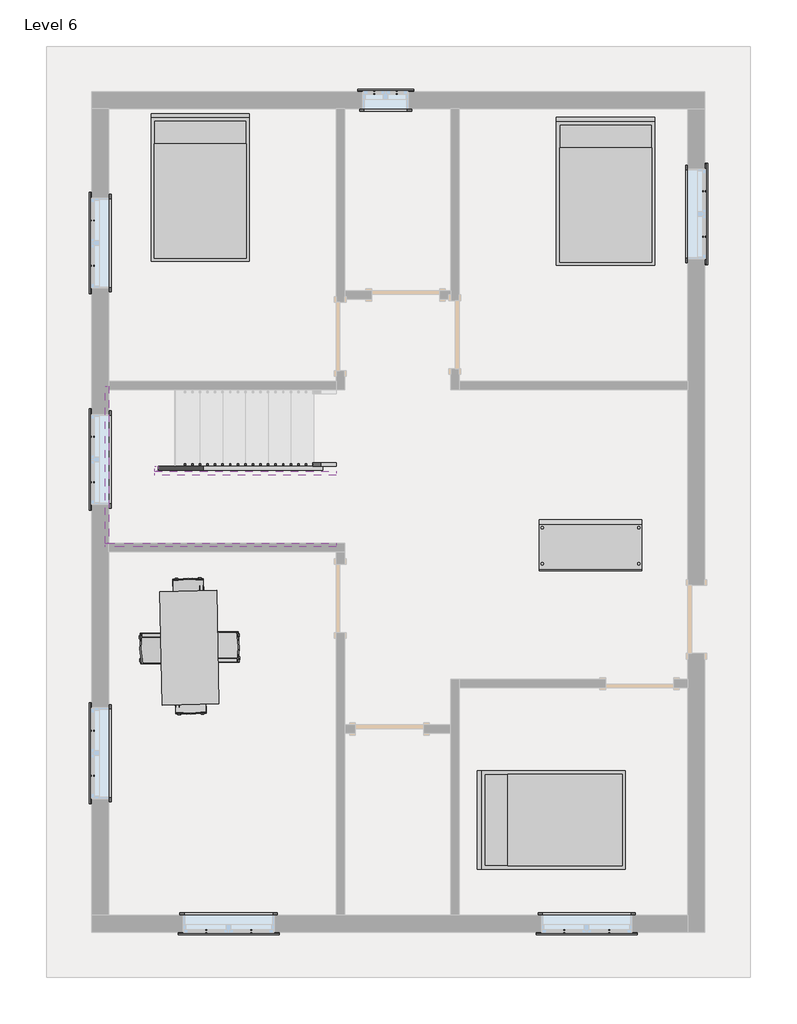
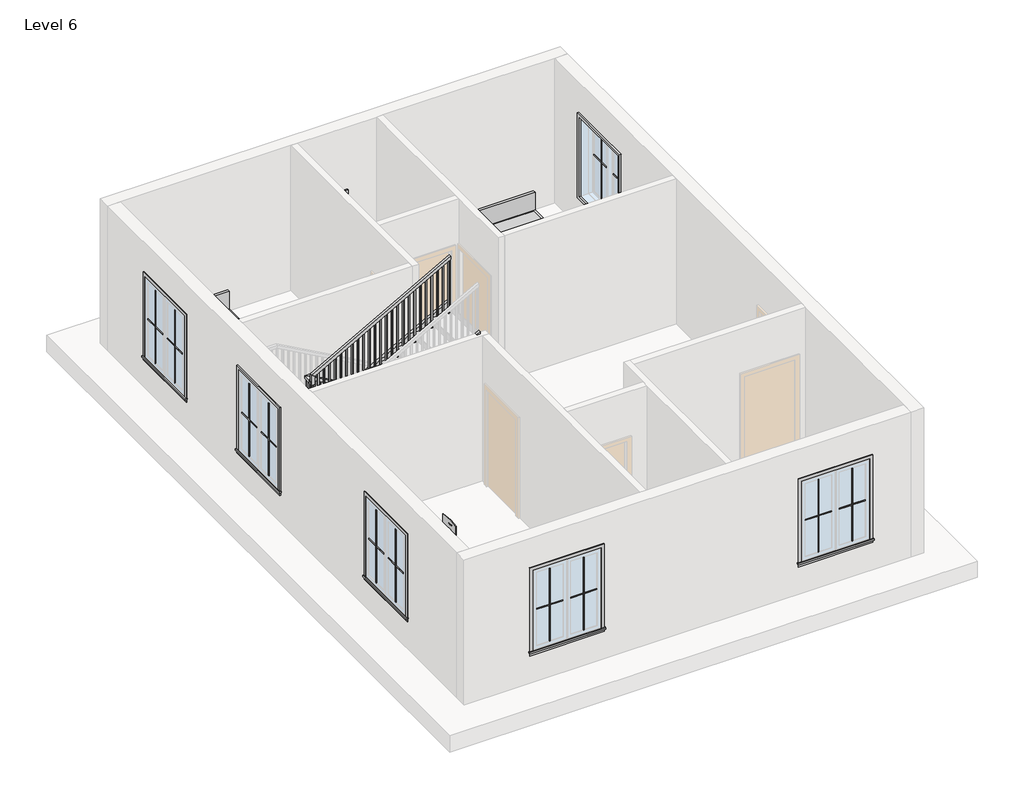
# One storey, part 2 of 2: 29 proxies, 6 members, 4 furniture elements, 1 railing.
"""IFC4 building model written with IfcOpenShell, lengths in millimetres."""

from ifc_helpers import new_model, si_unit, frame, origin, place, context, project, spatial, polyline, outline, extrude, faceted_brep, transform, mapped, element, save
from components import modern_coffee_table_17989_modern_coffee_table_17989_d3a860c8, muntin_pattern_2x2_muntin_pattern_2x2_6dad3731, muntin_pattern_2x2_muntin_pattern_2x2_a30a3345, muntin_pattern_2x2_muntin_pattern_2x2_53152e2c, muntin_pattern_2x2_muntin_pattern_2x2_e8f3e573, trim_window_exterior_flat_with_sill_92b9b949, trim_window_exterior_flat_with_sill_a665a915, trim_window_interior_flat_picture_frame_3bb882cf, trim_window_interior_flat_picture_frame_d485c387, bed_17739_bed_17739_15c61121, dining_table_w_chairs_11374_0cdfc61b

model = new_model("IFC4")

# Units and contexts
model_context = context("Model", 3, world=origin())
ifc_project = project(units=[si_unit("LENGTHUNIT", "METRE", prefix="MILLI")], contexts=[model_context])

# Site, building, storey
site = spatial("IfcSite", under=ifc_project)
building = spatial("IfcBuilding", under=site)
storey = spatial("IfcBuildingStorey", under=building, Name="Level 6", Elevation=15240.0)

# Proxies
placement = place(None, origin())
modern_coffee_table_17989_modern_coffee_table_17989_shape = modern_coffee_table_17989_modern_coffee_table_17989_d3a860c8(model_context)
element("IfcBuildingElementProxy", 1, Name="Modern_Coffee_Table_17989 : Modern_Coffee_Table_17989", ObjectType="Modern_Coffee_Table_17989 : Modern_Coffee_Table_17989", at=placement, inside=storey, context=model_context, shape_type="MappedRepresentation", body=[
    mapped(modern_coffee_table_17989_modern_coffee_table_17989_shape, transform((7937.5, 8234.1992646, 15240.0), x_axis=(1.0, 0.0, 0.0), y_axis=(0.0, 1.0, 0.0), z_axis=(0.0, 0.0, 1.0))),
])
muntin_pattern_2x2_muntin_pattern_2x2_shape = muntin_pattern_2x2_muntin_pattern_2x2_6dad3731(model_context)
element("IfcBuildingElementProxy", 2, Name="Muntin Pattern_2x2 : Muntin Pattern_2x2", ObjectType="Muntin Pattern_2x2 : Muntin Pattern_2x2", at=placement, inside=storey, context=model_context, shape_type="MappedRepresentation", body=[
    mapped(muntin_pattern_2x2_muntin_pattern_2x2_shape, transform((7961.3125, 2701.925, 16224.25), x_axis=(-1.0, 0.0, 0.0), y_axis=(0.0, -1.0, 0.0), z_axis=(0.0, 0.0, 1.0))),
])
element("IfcBuildingElementProxy", 3, Name="Muntin Pattern_2x2 : Muntin Pattern_2x2", ObjectType="Muntin Pattern_2x2 : Muntin Pattern_2x2", at=placement, inside=storey, context=model_context, shape_type="MappedRepresentation", body=[
    mapped(muntin_pattern_2x2_muntin_pattern_2x2_shape, transform((3154.3625, 2701.925, 16224.25), x_axis=(-1.0, 0.0, 0.0), y_axis=(0.0, -1.0, 0.0), z_axis=(0.0, 0.0, 1.0))),
])
element("IfcBuildingElementProxy", 4, Name="Muntin Pattern_2x2 : Muntin Pattern_2x2", ObjectType="Muntin Pattern_2x2 : Muntin Pattern_2x2", at=placement, inside=storey, context=model_context, shape_type="MappedRepresentation", body=[
    mapped(muntin_pattern_2x2_muntin_pattern_2x2_shape, transform((1025.525, 4789.4875, 16224.25), x_axis=(0.0, 1.0, 0.0), y_axis=(-1.0, 0.0, 0.0), z_axis=(0.0, 0.0, 1.0))),
])
element("IfcBuildingElementProxy", 5, Name="Muntin Pattern_2x2 : Muntin Pattern_2x2", ObjectType="Muntin Pattern_2x2 : Muntin Pattern_2x2", at=placement, inside=storey, context=model_context, shape_type="MappedRepresentation", body=[
    mapped(muntin_pattern_2x2_muntin_pattern_2x2_shape, transform((1025.525, 8732.8375, 16224.25), x_axis=(0.0, 1.0, 0.0), y_axis=(-1.0, 0.0, 0.0), z_axis=(0.0, 0.0, 1.0))),
])
element("IfcBuildingElementProxy", 6, Name="Muntin Pattern_2x2 : Muntin Pattern_2x2", ObjectType="Muntin Pattern_2x2 : Muntin Pattern_2x2", at=placement, inside=storey, context=model_context, shape_type="MappedRepresentation", body=[
    mapped(muntin_pattern_2x2_muntin_pattern_2x2_shape, transform((1025.525, 11637.9625, 16224.25), x_axis=(0.0, 1.0, 0.0), y_axis=(-1.0, 0.0, 0.0), z_axis=(0.0, 0.0, 1.0))),
])
element("IfcBuildingElementProxy", 7, Name="Muntin Pattern_2x2 : Muntin Pattern_2x2", ObjectType="Muntin Pattern_2x2 : Muntin Pattern_2x2", at=placement, inside=storey, context=model_context, shape_type="MappedRepresentation", body=[
    mapped(muntin_pattern_2x2_muntin_pattern_2x2_shape, transform((9236.075, 12634.9125, 16224.25), x_axis=(0.0, -1.0, 0.0), y_axis=(1.0, 0.0, 0.0), z_axis=(0.0, 0.0, 1.0))),
])
muntin_pattern_2x2_muntin_pattern_2x2_2_shape = muntin_pattern_2x2_muntin_pattern_2x2_a30a3345(model_context)
element("IfcBuildingElementProxy", 8, Name="Muntin Pattern_2x2 : Muntin Pattern_2x2", ObjectType="Muntin Pattern_2x2 : Muntin Pattern_2x2", at=placement, inside=storey, context=model_context, shape_type="MappedRepresentation", body=[
    mapped(muntin_pattern_2x2_muntin_pattern_2x2_2_shape, transform((7354.8875, 2701.925, 16224.25), x_axis=(1.0, 0.0, 0.0), y_axis=(0.0, 1.0, 0.0), z_axis=(0.0, 0.0, 1.0))),
])
element("IfcBuildingElementProxy", 9, Name="Muntin Pattern_2x2 : Muntin Pattern_2x2", ObjectType="Muntin Pattern_2x2 : Muntin Pattern_2x2", at=placement, inside=storey, context=model_context, shape_type="MappedRepresentation", body=[
    mapped(muntin_pattern_2x2_muntin_pattern_2x2_2_shape, transform((2547.9375, 2701.925, 16224.25), x_axis=(1.0, 0.0, 0.0), y_axis=(0.0, 1.0, 0.0), z_axis=(0.0, 0.0, 1.0))),
])
element("IfcBuildingElementProxy", 10, Name="Muntin Pattern_2x2 : Muntin Pattern_2x2", ObjectType="Muntin Pattern_2x2 : Muntin Pattern_2x2", at=placement, inside=storey, context=model_context, shape_type="MappedRepresentation", body=[
    mapped(muntin_pattern_2x2_muntin_pattern_2x2_2_shape, transform((1025.525, 5395.9125, 16224.25), x_axis=(0.0, -1.0, 0.0), y_axis=(1.0, 0.0, 0.0), z_axis=(0.0, 0.0, 1.0))),
])
element("IfcBuildingElementProxy", 11, Name="Muntin Pattern_2x2 : Muntin Pattern_2x2", ObjectType="Muntin Pattern_2x2 : Muntin Pattern_2x2", at=placement, inside=storey, context=model_context, shape_type="MappedRepresentation", body=[
    mapped(muntin_pattern_2x2_muntin_pattern_2x2_2_shape, transform((1025.525, 9339.2625, 16224.25), x_axis=(0.0, -1.0, 0.0), y_axis=(1.0, 0.0, 0.0), z_axis=(0.0, 0.0, 1.0))),
])
element("IfcBuildingElementProxy", 12, Name="Muntin Pattern_2x2 : Muntin Pattern_2x2", ObjectType="Muntin Pattern_2x2 : Muntin Pattern_2x2", at=placement, inside=storey, context=model_context, shape_type="MappedRepresentation", body=[
    mapped(muntin_pattern_2x2_muntin_pattern_2x2_2_shape, transform((1025.525, 12244.3875, 16224.25), x_axis=(0.0, -1.0, 0.0), y_axis=(1.0, 0.0, 0.0), z_axis=(0.0, 0.0, 1.0))),
])
element("IfcBuildingElementProxy", 13, Name="Muntin Pattern_2x2 : Muntin Pattern_2x2", ObjectType="Muntin Pattern_2x2 : Muntin Pattern_2x2", at=placement, inside=storey, context=model_context, shape_type="MappedRepresentation", body=[
    mapped(muntin_pattern_2x2_muntin_pattern_2x2_2_shape, transform((9236.075, 12028.4875, 16224.25), x_axis=(0.0, 1.0, 0.0), y_axis=(-1.0, 0.0, 0.0), z_axis=(0.0, 0.0, 1.0))),
])
muntin_pattern_2x2_muntin_pattern_2x2_3_shape = muntin_pattern_2x2_muntin_pattern_2x2_53152e2c(model_context)
element("IfcBuildingElementProxy", 14, Name="Muntin Pattern_2x2 : Muntin Pattern_2x2", ObjectType="Muntin Pattern_2x2 : Muntin Pattern_2x2", at=placement, inside=storey, context=model_context, shape_type="MappedRepresentation", body=[
    mapped(muntin_pattern_2x2_muntin_pattern_2x2_3_shape, transform((4808.5375, 13960.475, 16224.25), x_axis=(1.0, 0.0, 0.0), y_axis=(0.0, 1.0, 0.0), z_axis=(0.0, 0.0, 1.0))),
])
muntin_pattern_2x2_muntin_pattern_2x2_4_shape = muntin_pattern_2x2_muntin_pattern_2x2_e8f3e573(model_context)
element("IfcBuildingElementProxy", 15, Name="Muntin Pattern_2x2 : Muntin Pattern_2x2", ObjectType="Muntin Pattern_2x2 : Muntin Pattern_2x2", at=placement, inside=storey, context=model_context, shape_type="MappedRepresentation", body=[
    mapped(muntin_pattern_2x2_muntin_pattern_2x2_4_shape, transform((5110.1625, 13960.475, 16224.25), x_axis=(-1.0, 0.0, 0.0), y_axis=(0.0, -1.0, 0.0), z_axis=(0.0, 0.0, 1.0))),
])
trim_window_exterior_flat_with_sill_shape = trim_window_exterior_flat_with_sill_92b9b949(model_context)
element("IfcBuildingElementProxy", 16, Name="Trim-Window-Exterior-Flat : with Sill", ObjectType="Trim-Window-Exterior-Flat : with Sill", at=placement, inside=storey, context=model_context, shape_type="MappedRepresentation", body=[
    mapped(trim_window_exterior_flat_with_sill_shape, transform((7658.1, 2692.4, 17678.4), x_axis=(1.0, 0.0, 0.0), y_axis=(0.0, 0.0, 1.0), z_axis=(0.0, -1.0, 0.0))),
])
element("IfcBuildingElementProxy", 17, Name="Trim-Window-Exterior-Flat : with Sill", ObjectType="Trim-Window-Exterior-Flat : with Sill", at=placement, inside=storey, context=model_context, shape_type="MappedRepresentation", body=[
    mapped(trim_window_exterior_flat_with_sill_shape, transform((2851.15, 2692.4, 17678.4), x_axis=(1.0, 0.0, 0.0), y_axis=(0.0, 0.0, 1.0), z_axis=(0.0, -1.0, 0.0))),
])
element("IfcBuildingElementProxy", 18, Name="Trim-Window-Exterior-Flat : with Sill", ObjectType="Trim-Window-Exterior-Flat : with Sill", at=placement, inside=storey, context=model_context, shape_type="MappedRepresentation", body=[
    mapped(trim_window_exterior_flat_with_sill_shape, transform((1016.0, 5092.7, 17678.4), x_axis=(0.0, -1.0, 0.0), y_axis=(0.0, 0.0, 1.0), z_axis=(-1.0, 0.0, 0.0))),
])
element("IfcBuildingElementProxy", 19, Name="Trim-Window-Exterior-Flat : with Sill", ObjectType="Trim-Window-Exterior-Flat : with Sill", at=placement, inside=storey, context=model_context, shape_type="MappedRepresentation", body=[
    mapped(trim_window_exterior_flat_with_sill_shape, transform((1016.0, 9036.05, 17678.4), x_axis=(0.0, -1.0, 0.0), y_axis=(0.0, 0.0, 1.0), z_axis=(-1.0, 0.0, 0.0))),
])
element("IfcBuildingElementProxy", 20, Name="Trim-Window-Exterior-Flat : with Sill", ObjectType="Trim-Window-Exterior-Flat : with Sill", at=placement, inside=storey, context=model_context, shape_type="MappedRepresentation", body=[
    mapped(trim_window_exterior_flat_with_sill_shape, transform((1016.0, 11941.175, 17678.4), x_axis=(0.0, -1.0, 0.0), y_axis=(0.0, 0.0, 1.0), z_axis=(-1.0, 0.0, 0.0))),
])
element("IfcBuildingElementProxy", 21, Name="Trim-Window-Exterior-Flat : with Sill", ObjectType="Trim-Window-Exterior-Flat : with Sill", at=placement, inside=storey, context=model_context, shape_type="MappedRepresentation", body=[
    mapped(trim_window_exterior_flat_with_sill_shape, transform((9245.6, 12331.7, 17678.4), x_axis=(0.0, 1.0, 0.0), y_axis=(0.0, 0.0, 1.0), z_axis=(1.0, 0.0, 0.0))),
])
trim_window_exterior_flat_with_sill_2_shape = trim_window_exterior_flat_with_sill_a665a915(model_context)
element("IfcBuildingElementProxy", 22, Name="Trim-Window-Exterior-Flat : with Sill", ObjectType="Trim-Window-Exterior-Flat : with Sill", at=placement, inside=storey, context=model_context, shape_type="MappedRepresentation", body=[
    mapped(trim_window_exterior_flat_with_sill_2_shape, transform((4959.35, 13970.0, 17068.8), x_axis=(-1.0, 0.0, 0.0), y_axis=(0.0, 0.0, 1.0), z_axis=(0.0, 1.0, 0.0))),
])
trim_window_interior_flat_picture_frame_shape = trim_window_interior_flat_picture_frame_3bb882cf(model_context)
element("IfcBuildingElementProxy", 23, Name="Trim-Window-Interior-Flat : Picture Frame", ObjectType="Trim-Window-Interior-Flat : Picture Frame", at=placement, inside=storey, context=model_context, shape_type="MappedRepresentation", body=[
    mapped(trim_window_interior_flat_picture_frame_shape, transform((7658.1, 2921.0, 17678.4), x_axis=(-1.0, 0.0, 0.0), y_axis=(0.0, 0.0, 1.0), z_axis=(0.0, 1.0, 0.0))),
])
element("IfcBuildingElementProxy", 24, Name="Trim-Window-Interior-Flat : Picture Frame", ObjectType="Trim-Window-Interior-Flat : Picture Frame", at=placement, inside=storey, context=model_context, shape_type="MappedRepresentation", body=[
    mapped(trim_window_interior_flat_picture_frame_shape, transform((2851.15, 2921.0, 17678.4), x_axis=(-1.0, 0.0, 0.0), y_axis=(0.0, 0.0, 1.0), z_axis=(0.0, 1.0, 0.0))),
])
element("IfcBuildingElementProxy", 25, Name="Trim-Window-Interior-Flat : Picture Frame", ObjectType="Trim-Window-Interior-Flat : Picture Frame", at=placement, inside=storey, context=model_context, shape_type="MappedRepresentation", body=[
    mapped(trim_window_interior_flat_picture_frame_shape, transform((1244.6, 5092.7, 17678.4), x_axis=(0.0, 1.0, 0.0), y_axis=(0.0, 0.0, 1.0), z_axis=(1.0, 0.0, 0.0))),
])
element("IfcBuildingElementProxy", 26, Name="Trim-Window-Interior-Flat : Picture Frame", ObjectType="Trim-Window-Interior-Flat : Picture Frame", at=placement, inside=storey, context=model_context, shape_type="MappedRepresentation", body=[
    mapped(trim_window_interior_flat_picture_frame_shape, transform((1244.6, 9036.05, 17678.4), x_axis=(0.0, 1.0, 0.0), y_axis=(0.0, 0.0, 1.0), z_axis=(1.0, 0.0, 0.0))),
])
element("IfcBuildingElementProxy", 27, Name="Trim-Window-Interior-Flat : Picture Frame", ObjectType="Trim-Window-Interior-Flat : Picture Frame", at=placement, inside=storey, context=model_context, shape_type="MappedRepresentation", body=[
    mapped(trim_window_interior_flat_picture_frame_shape, transform((1244.6, 11941.175, 17678.4), x_axis=(0.0, 1.0, 0.0), y_axis=(0.0, 0.0, 1.0), z_axis=(1.0, 0.0, 0.0))),
])
element("IfcBuildingElementProxy", 28, Name="Trim-Window-Interior-Flat : Picture Frame", ObjectType="Trim-Window-Interior-Flat : Picture Frame", at=placement, inside=storey, context=model_context, shape_type="MappedRepresentation", body=[
    mapped(trim_window_interior_flat_picture_frame_shape, transform((9017.0, 12331.7, 17678.4), x_axis=(0.0, -1.0, 0.0), y_axis=(0.0, 0.0, 1.0), z_axis=(-1.0, 0.0, 0.0))),
])
trim_window_interior_flat_picture_frame_2_shape = trim_window_interior_flat_picture_frame_d485c387(model_context)
element("IfcBuildingElementProxy", 29, Name="Trim-Window-Interior-Flat : Picture Frame", ObjectType="Trim-Window-Interior-Flat : Picture Frame", at=placement, inside=storey, context=model_context, shape_type="MappedRepresentation", body=[
    mapped(trim_window_interior_flat_picture_frame_2_shape, transform((4959.35, 13741.4, 17068.8), x_axis=(1.0, 0.0, 0.0), y_axis=(0.0, 0.0, 1.0), z_axis=(0.0, -1.0, 0.0))),
])

# Furniture
bed_17739_bed_17739_shape = bed_17739_bed_17739_15c61121(model_context)
element("IfcFurniture", 30, ObjectType="Bed_17739 : Bed_17739", at=placement, inside=storey, context=model_context, shape_type="MappedRepresentation", body=[
    mapped(bed_17739_bed_17739_shape, transform((2470.15, 12661.9, 15240.0), x_axis=(1.0, 0.0, 0.0), y_axis=(0.0, 1.0, 0.0), z_axis=(0.0, 0.0, 1.0))),
])
element("IfcFurniture", 31, ObjectType="Bed_17739 : Bed_17739", at=placement, inside=storey, context=model_context, shape_type="MappedRepresentation", body=[
    mapped(bed_17739_bed_17739_shape, transform((7912.1, 12611.1, 15240.0), x_axis=(1.0, 0.0, 0.0), y_axis=(0.0, 1.0, 0.0), z_axis=(0.0, 0.0, 1.0))),
])
element("IfcFurniture", 32, ObjectType="Bed_17739 : Bed_17739", at=placement, inside=storey, context=model_context, shape_type="MappedRepresentation", body=[
    mapped(bed_17739_bed_17739_shape, transform((7207.25, 4197.35, 15240.0), x_axis=(0.0, 1.0, 0.0), y_axis=(-1.0, 0.0, 0.0), z_axis=(0.0, 0.0, 1.0))),
])
dining_table_w_chairs_11374_shape = dining_table_w_chairs_11374_0cdfc61b(model_context)
element("IfcFurniture", 33, ObjectType="Dining_Table_w_Chairs_11374", at=placement, inside=storey, context=model_context, shape_type="MappedRepresentation", body=[
    mapped(dining_table_w_chairs_11374_shape, transform((2420.6366388, 6492.5326572, 15240.0), x_axis=(-0.019560245774115807, 0.9998086800909743, 0.0), y_axis=(-0.9998086800909743, -0.019560245774115807, 0.0), z_axis=(0.0, 0.0, 1.0))),
])

# Members
element("IfcMember", 34, ObjectType="Stringer - 2\" Width", at=placement, inside=storey, context=model_context, shape_type="SweptSolid", body=[
    extrude(outline(polyline([(15240.0, 4295.1355783), (15447.5983948, 4295.1355783), (16774.0428392, 1907.5355783), (16425.3641651, 1907.5355783), (15240.0, 4041.1910755), (15240.0, 4295.1355783)])), frame((0.0, 8893.8068332, 0.0), z_axis=(0.0, 1.0, 0.0), x_axis=(0.0, 0.0, 1.0)), (0.0, 0.0, 1.0), 50.8),
])
element("IfcMember", 35, ObjectType="Stringer - 2\" Width", at=placement, inside=storey, context=model_context, shape_type="SweptSolid", body=[
    extrude(outline(polyline([(1856.7355783, 8944.6068332), (1907.5355783, 8944.6068332), (1907.5355783, 8877.3), (1856.7355783, 8877.3), (1856.7355783, 8944.6068332)])), frame((0.0, 0.0, 16535.4), z_axis=(0.0, 0.0, 1.0), x_axis=(1.0, 0.0, 0.0)), (0.0, 0.0, 1.0), 304.8),
])
element("IfcMember", 36, ObjectType="Stringer - 2\" Width", at=placement, inside=storey, context=model_context, shape_type="SweptSolid", body=[
    extrude(outline(polyline([(16971.5983948, 1856.7355783), (16622.9197207, 1856.7355783), (17977.5863873, 4295.1355783), (18326.2650614, 4295.1355783), (16971.5983948, 1856.7355783)])), frame((0.0, 8826.5, 0.0), z_axis=(0.0, 1.0, 0.0), x_axis=(0.0, 0.0, 1.0)), (0.0, 0.0, 1.0), 50.8),
])
element("IfcMember", 37, ObjectType="Stringer - 2\" Width", at=placement, inside=storey, context=model_context, shape_type="SweptSolid", body=[
    extrude(outline(polyline([(15240.0, 4295.1355783), (15447.5983948, 4295.1355783), (16840.2, 1788.4526889), (16840.2, 1244.6), (16793.6617086, 1244.6), (15240.0, 4041.1910755), (15240.0, 4295.1355783)])), frame((0.0, 9969.5, 0.0), z_axis=(0.0, 1.0, 0.0), x_axis=(0.0, 0.0, 1.0)), (0.0, 0.0, 1.0), 50.8),
])
element("IfcMember", 38, ObjectType="Stringer - 2\" Width", at=placement, inside=storey, context=model_context, shape_type="SweptSolid", body=[
    extrude(outline(polyline([(1193.8, 10020.3), (1244.6, 10020.3), (1244.6, 7912.1), (1193.8, 7912.1), (1193.8, 10020.3)])), frame((0.0, 0.0, 16535.4), z_axis=(0.0, 0.0, 1.0), x_axis=(1.0, 0.0, 0.0)), (0.0, 0.0, 1.0), 304.8),
])
element("IfcMember", 39, ObjectType="Stringer - 2\" Width", at=placement, inside=storey, context=model_context, shape_type="SweptSolid", body=[
    extrude(outline(polyline([(16603.3008513, 1193.8), (16535.4, 1193.8), (16535.4, 1699.2000811), (17977.5863873, 4295.1355783), (18326.2650614, 4295.1355783), (16603.3008513, 1193.8)])), frame((0.0, 7861.3, 0.0), z_axis=(0.0, 1.0, 0.0), x_axis=(0.0, 0.0, 1.0)), (0.0, 0.0, 1.0), 50.8),
])

# Railing
element("IfcRailing", 40, ObjectType="Handrail - Rectangular", at=placement, inside=storey, context=model_context, shape_type="SolidModel", body=[
    faceted_brep([(4295.1355783, 8944.6068332, 16323.7333333), (4295.1355783, 8944.6068332, 16265.620221), (4295.1355783, 8995.4068332, 16265.620221), (4295.1355783, 8995.4068332, 16323.7333333), (1932.9355783, 8944.6068332, 17636.0666667), (1882.1355783, 8944.6068332, 17606.1757765), (1882.1355783, 8995.4068332, 17606.1757765), (1932.9355783, 8995.4068332, 17636.0666667), (1932.9355783, 8944.6068332, 17678.4), (1882.1355783, 8944.6068332, 17627.6), (1882.1355783, 8995.4068332, 17627.6), (1932.9355783, 8995.4068332, 17678.4), (1856.7355783, 8944.6068332, 17678.4), (1856.7355783, 8944.6068332, 17627.6), (1805.9355783, 8995.4068332, 17627.6), (1805.9355783, 8995.4068332, 17678.4), (1856.7355783, 8868.4068332, 17678.4), (1856.7355783, 8868.4068332, 17627.6), (1805.9355783, 8868.4068332, 17627.6), (1805.9355783, 8868.4068332, 17678.4), (1856.7355783, 8826.5, 17678.4), (1805.9355783, 8826.5, 17678.4), (1805.9355783, 8775.7, 17627.6), (1856.7355783, 8775.7, 17627.6)], [[[0, 1, 2, 3]], [[1, 0, 4, 5]], [[2, 1, 5, 6]], [[3, 2, 6, 7]], [[0, 3, 7, 4]], [[5, 4, 8, 9]], [[6, 5, 9, 10]], [[7, 6, 10, 11]], [[4, 7, 11, 8]], [[9, 8, 12, 13]], [[10, 9, 13, 14]], [[11, 10, 14, 15]], [[8, 11, 15, 12]], [[13, 12, 16, 17]], [[14, 13, 17, 18]], [[15, 14, 18, 19]], [[12, 15, 19, 16]], [[20, 21, 22, 23]], [[17, 16, 20, 23]], [[18, 17, 23, 22]], [[19, 18, 22, 21]], [[16, 19, 21, 20]]]),
    faceted_brep([(1856.7355783, 8826.5, 17678.4), (1856.7355783, 8775.7, 17627.6), (1805.9355783, 8775.7, 17627.6), (1805.9355783, 8826.5, 17678.4), (1856.7355783, 8826.5, 17789.620221), (1805.9355783, 8826.5, 17819.5111111), (1805.9355783, 8775.7, 17819.5111111), (1856.7355783, 8775.7, 17789.620221)], [[[0, 1, 2, 3]], [[4, 5, 6, 7]], [[1, 0, 4, 7]], [[2, 1, 7, 6]], [[3, 2, 6, 5]], [[0, 3, 5, 4]]]),
    faceted_brep([(1805.9355783, 8826.5, 17819.5111111), (1856.7355783, 8826.5, 17789.620221), (1856.7355783, 8775.7, 17789.620221), (1805.9355783, 8775.7, 17819.5111111), (4295.1355783, 8826.5, 19202.4), (4295.1355783, 8775.7, 19202.4), (4295.1355783, 8775.7, 19144.2868876), (4295.1355783, 8826.5, 19144.2868876)], [[[0, 1, 2, 3]], [[4, 5, 6, 7]], [[1, 0, 4, 7]], [[2, 1, 7, 6]], [[3, 2, 6, 5]], [[0, 3, 5, 4]]]),
    extrude(outline(polyline([(19124.8841099, 4260.2105783), (18118.6666667, 4260.2105783), (18118.6666667, 4279.2605783), (19135.4674432, 4279.2605783), (19124.8841099, 4260.2105783)])), frame((0.0, 8791.575, 0.0), z_axis=(0.0, 1.0, 0.0), x_axis=(0.0, 0.0, 1.0)), (0.0, 0.0, 1.0), 19.05),
    extrude(outline(polyline([(19068.4396654, 4158.6105783), (18118.6666667, 4158.6105783), (18118.6666667, 4177.6605783), (19079.0229988, 4177.6605783), (19068.4396654, 4158.6105783)])), frame((0.0, 8791.575, 0.0), z_axis=(0.0, 1.0, 0.0), x_axis=(0.0, 0.0, 1.0)), (0.0, 0.0, 1.0), 19.05),
    extrude(outline(polyline([(19011.995221, 4057.0105783), (18118.6666667, 4057.0105783), (18118.6666667, 4076.0605783), (19022.5785543, 4076.0605783), (19011.995221, 4057.0105783)])), frame((0.0, 8791.575, 0.0), z_axis=(0.0, 1.0, 0.0), x_axis=(0.0, 0.0, 1.0)), (0.0, 0.0, 1.0), 19.05),
    extrude(outline(polyline([(18955.5507765, 3955.4105783), (17949.3333333, 3955.4105783), (17949.3333333, 3974.4605783), (18966.1341099, 3974.4605783), (18955.5507765, 3955.4105783)])), frame((0.0, 8791.575, 0.0), z_axis=(0.0, 1.0, 0.0), x_axis=(0.0, 0.0, 1.0)), (0.0, 0.0, 1.0), 19.05),
    extrude(outline(polyline([(18899.1063321, 3853.8105783), (17949.3333333, 3853.8105783), (17949.3333333, 3872.8605783), (18909.6896654, 3872.8605783), (18899.1063321, 3853.8105783)])), frame((0.0, 8791.575, 0.0), z_axis=(0.0, 1.0, 0.0), x_axis=(0.0, 0.0, 1.0)), (0.0, 0.0, 1.0), 19.05),
    extrude(outline(polyline([(18842.6618876, 3752.2105783), (17949.3333333, 3752.2105783), (17949.3333333, 3771.2605783), (18853.245221, 3771.2605783), (18842.6618876, 3752.2105783)])), frame((0.0, 8791.575, 0.0), z_axis=(0.0, 1.0, 0.0), x_axis=(0.0, 0.0, 1.0)), (0.0, 0.0, 1.0), 19.05),
    extrude(outline(polyline([(18786.2174432, 3650.6105783), (17780.0, 3650.6105783), (17780.0, 3669.6605783), (18796.8007765, 3669.6605783), (18786.2174432, 3650.6105783)])), frame((0.0, 8791.575, 0.0), z_axis=(0.0, 1.0, 0.0), x_axis=(0.0, 0.0, 1.0)), (0.0, 0.0, 1.0), 19.05),
    extrude(outline(polyline([(18729.7729988, 3549.0105783), (17780.0, 3549.0105783), (17780.0, 3568.0605783), (18740.3563321, 3568.0605783), (18729.7729988, 3549.0105783)])), frame((0.0, 8791.575, 0.0), z_axis=(0.0, 1.0, 0.0), x_axis=(0.0, 0.0, 1.0)), (0.0, 0.0, 1.0), 19.05),
    extrude(outline(polyline([(18673.3285543, 3447.4105783), (17780.0, 3447.4105783), (17780.0, 3466.4605783), (18683.9118876, 3466.4605783), (18673.3285543, 3447.4105783)])), frame((0.0, 8791.575, 0.0), z_axis=(0.0, 1.0, 0.0), x_axis=(0.0, 0.0, 1.0)), (0.0, 0.0, 1.0), 19.05),
    extrude(outline(polyline([(18616.8841099, 3345.8105783), (17610.6666667, 3345.8105783), (17610.6666667, 3364.8605783), (18627.4674432, 3364.8605783), (18616.8841099, 3345.8105783)])), frame((0.0, 8791.575, 0.0), z_axis=(0.0, 1.0, 0.0), x_axis=(0.0, 0.0, 1.0)), (0.0, 0.0, 1.0), 19.05),
    extrude(outline(polyline([(18560.4396654, 3244.2105783), (17610.6666667, 3244.2105783), (17610.6666667, 3263.2605783), (18571.0229988, 3263.2605783), (18560.4396654, 3244.2105783)])), frame((0.0, 8791.575, 0.0), z_axis=(0.0, 1.0, 0.0), x_axis=(0.0, 0.0, 1.0)), (0.0, 0.0, 1.0), 19.05),
    extrude(outline(polyline([(18503.995221, 3142.6105783), (17610.6666667, 3142.6105783), (17610.6666667, 3161.6605783), (18514.5785543, 3161.6605783), (18503.995221, 3142.6105783)])), frame((0.0, 8791.575, 0.0), z_axis=(0.0, 1.0, 0.0), x_axis=(0.0, 0.0, 1.0)), (0.0, 0.0, 1.0), 19.05),
    extrude(outline(polyline([(18447.5507765, 3041.0105783), (17441.3333333, 3041.0105783), (17441.3333333, 3060.0605783), (18458.1341099, 3060.0605783), (18447.5507765, 3041.0105783)])), frame((0.0, 8791.575, 0.0), z_axis=(0.0, 1.0, 0.0), x_axis=(0.0, 0.0, 1.0)), (0.0, 0.0, 1.0), 19.05),
    extrude(outline(polyline([(18391.1063321, 2939.4105783), (17441.3333333, 2939.4105783), (17441.3333333, 2958.4605783), (18401.6896654, 2958.4605783), (18391.1063321, 2939.4105783)])), frame((0.0, 8791.575, 0.0), z_axis=(0.0, 1.0, 0.0), x_axis=(0.0, 0.0, 1.0)), (0.0, 0.0, 1.0), 19.05),
    extrude(outline(polyline([(18334.6618876, 2837.8105783), (17441.3333333, 2837.8105783), (17441.3333333, 2856.8605783), (18345.245221, 2856.8605783), (18334.6618876, 2837.8105783)])), frame((0.0, 8791.575, 0.0), z_axis=(0.0, 1.0, 0.0), x_axis=(0.0, 0.0, 1.0)), (0.0, 0.0, 1.0), 19.05),
    extrude(outline(polyline([(18278.2174432, 2736.2105783), (17272.0, 2736.2105783), (17272.0, 2755.2605783), (18288.8007765, 2755.2605783), (18278.2174432, 2736.2105783)])), frame((0.0, 8791.575, 0.0), z_axis=(0.0, 1.0, 0.0), x_axis=(0.0, 0.0, 1.0)), (0.0, 0.0, 1.0), 19.05),
    extrude(outline(polyline([(18221.7729988, 2634.6105783), (17272.0, 2634.6105783), (17272.0, 2653.6605783), (18232.3563321, 2653.6605783), (18221.7729988, 2634.6105783)])), frame((0.0, 8791.575, 0.0), z_axis=(0.0, 1.0, 0.0), x_axis=(0.0, 0.0, 1.0)), (0.0, 0.0, 1.0), 19.05),
    extrude(outline(polyline([(18165.3285543, 2533.0105783), (17272.0, 2533.0105783), (17272.0, 2552.0605783), (18175.9118876, 2552.0605783), (18165.3285543, 2533.0105783)])), frame((0.0, 8791.575, 0.0), z_axis=(0.0, 1.0, 0.0), x_axis=(0.0, 0.0, 1.0)), (0.0, 0.0, 1.0), 19.05),
    extrude(outline(polyline([(18108.8841099, 2431.4105783), (17102.6666667, 2431.4105783), (17102.6666667, 2450.4605783), (18119.4674432, 2450.4605783), (18108.8841099, 2431.4105783)])), frame((0.0, 8791.575, 0.0), z_axis=(0.0, 1.0, 0.0), x_axis=(0.0, 0.0, 1.0)), (0.0, 0.0, 1.0), 19.05),
    extrude(outline(polyline([(18052.4396654, 2329.8105783), (17102.6666667, 2329.8105783), (17102.6666667, 2348.8605783), (18063.0229988, 2348.8605783), (18052.4396654, 2329.8105783)])), frame((0.0, 8791.575, 0.0), z_axis=(0.0, 1.0, 0.0), x_axis=(0.0, 0.0, 1.0)), (0.0, 0.0, 1.0), 19.05),
    extrude(outline(polyline([(17995.995221, 2228.2105783), (17102.6666667, 2228.2105783), (17102.6666667, 2247.2605783), (18006.5785543, 2247.2605783), (17995.995221, 2228.2105783)])), frame((0.0, 8791.575, 0.0), z_axis=(0.0, 1.0, 0.0), x_axis=(0.0, 0.0, 1.0)), (0.0, 0.0, 1.0), 19.05),
    extrude(outline(polyline([(17939.5507765, 2126.6105783), (16933.3333333, 2126.6105783), (16933.3333333, 2145.6605783), (17950.1341099, 2145.6605783), (17939.5507765, 2126.6105783)])), frame((0.0, 8791.575, 0.0), z_axis=(0.0, 1.0, 0.0), x_axis=(0.0, 0.0, 1.0)), (0.0, 0.0, 1.0), 19.05),
    extrude(outline(polyline([(17883.1063321, 2025.0105783), (16933.3333333, 2025.0105783), (16933.3333333, 2044.0605783), (17893.6896654, 2044.0605783), (17883.1063321, 2025.0105783)])), frame((0.0, 8791.575, 0.0), z_axis=(0.0, 1.0, 0.0), x_axis=(0.0, 0.0, 1.0)), (0.0, 0.0, 1.0), 19.05),
    extrude(outline(polyline([(17826.6618876, 1923.4105783), (16933.3333333, 1923.4105783), (16933.3333333, 1942.4605783), (17837.245221, 1942.4605783), (17826.6618876, 1923.4105783)])), frame((0.0, 8791.575, 0.0), z_axis=(0.0, 1.0, 0.0), x_axis=(0.0, 0.0, 1.0)), (0.0, 0.0, 1.0), 19.05),
    extrude(outline(polyline([(1840.8605783, 8877.9318332), (1840.8605783, 8858.8818332), (1821.8105783, 8858.8818332), (1821.8105783, 8877.9318332), (1840.8605783, 8877.9318332)])), frame((0.0, 0.0, 16764.0), z_axis=(0.0, 0.0, 1.0), x_axis=(1.0, 0.0, 0.0)), (0.0, 0.0, 1.0), 863.6),
    extrude(outline(polyline([(1866.2605783, 8960.4818332), (1847.2105783, 8960.4818332), (1847.2105783, 8979.5318332), (1866.2605783, 8979.5318332), (1866.2605783, 8960.4818332)])), frame((0.0, 0.0, 16764.0), z_axis=(0.0, 0.0, 1.0), x_axis=(1.0, 0.0, 0.0)), (0.0, 0.0, 1.0), 863.6),
    extrude(outline(polyline([(17569.1341099, 1948.8105783), (16594.6666667, 1948.8105783), (16594.6666667, 1967.8605783), (17558.5507765, 1967.8605783), (17569.1341099, 1948.8105783)])), frame((0.0, 8960.4818332, 0.0), z_axis=(0.0, 1.0, 0.0), x_axis=(0.0, 0.0, 1.0)), (0.0, 0.0, 1.0), 19.05),
    extrude(outline(polyline([(17512.6896654, 2050.4105783), (16594.6666667, 2050.4105783), (16594.6666667, 2069.4605783), (17502.1063321, 2069.4605783), (17512.6896654, 2050.4105783)])), frame((0.0, 8960.4818332, 0.0), z_axis=(0.0, 1.0, 0.0), x_axis=(0.0, 0.0, 1.0)), (0.0, 0.0, 1.0), 19.05),
    extrude(outline(polyline([(17456.245221, 2152.0105783), (16594.6666667, 2152.0105783), (16594.6666667, 2171.0605783), (17445.6618876, 2171.0605783), (17456.245221, 2152.0105783)])), frame((0.0, 8960.4818332, 0.0), z_axis=(0.0, 1.0, 0.0), x_axis=(0.0, 0.0, 1.0)), (0.0, 0.0, 1.0), 19.05),
    extrude(outline(polyline([(17399.8007765, 2253.6105783), (16425.3333333, 2253.6105783), (16425.3333333, 2272.6605783), (17389.2174432, 2272.6605783), (17399.8007765, 2253.6105783)])), frame((0.0, 8960.4818332, 0.0), z_axis=(0.0, 1.0, 0.0), x_axis=(0.0, 0.0, 1.0)), (0.0, 0.0, 1.0), 19.05),
    extrude(outline(polyline([(17343.3563321, 2355.2105783), (16425.3333333, 2355.2105783), (16425.3333333, 2374.2605783), (17332.7729988, 2374.2605783), (17343.3563321, 2355.2105783)])), frame((0.0, 8960.4818332, 0.0), z_axis=(0.0, 1.0, 0.0), x_axis=(0.0, 0.0, 1.0)), (0.0, 0.0, 1.0), 19.05),
    extrude(outline(polyline([(17286.9118876, 2456.8105783), (16425.3333333, 2456.8105783), (16425.3333333, 2475.8605783), (17276.3285543, 2475.8605783), (17286.9118876, 2456.8105783)])), frame((0.0, 8960.4818332, 0.0), z_axis=(0.0, 1.0, 0.0), x_axis=(0.0, 0.0, 1.0)), (0.0, 0.0, 1.0), 19.05),
    extrude(outline(polyline([(17230.4674432, 2558.4105783), (16256.0, 2558.4105783), (16256.0, 2577.4605783), (17219.8841099, 2577.4605783), (17230.4674432, 2558.4105783)])), frame((0.0, 8960.4818332, 0.0), z_axis=(0.0, 1.0, 0.0), x_axis=(0.0, 0.0, 1.0)), (0.0, 0.0, 1.0), 19.05),
    extrude(outline(polyline([(17174.0229988, 2660.0105783), (16256.0, 2660.0105783), (16256.0, 2679.0605783), (17163.4396654, 2679.0605783), (17174.0229988, 2660.0105783)])), frame((0.0, 8960.4818332, 0.0), z_axis=(0.0, 1.0, 0.0), x_axis=(0.0, 0.0, 1.0)), (0.0, 0.0, 1.0), 19.05),
    extrude(outline(polyline([(17117.5785543, 2761.6105783), (16256.0, 2761.6105783), (16256.0, 2780.6605783), (17106.995221, 2780.6605783), (17117.5785543, 2761.6105783)])), frame((0.0, 8960.4818332, 0.0), z_axis=(0.0, 1.0, 0.0), x_axis=(0.0, 0.0, 1.0)), (0.0, 0.0, 1.0), 19.05),
    extrude(outline(polyline([(17061.1341099, 2863.2105783), (16086.6666667, 2863.2105783), (16086.6666667, 2882.2605783), (17050.5507765, 2882.2605783), (17061.1341099, 2863.2105783)])), frame((0.0, 8960.4818332, 0.0), z_axis=(0.0, 1.0, 0.0), x_axis=(0.0, 0.0, 1.0)), (0.0, 0.0, 1.0), 19.05),
    extrude(outline(polyline([(17004.6896654, 2964.8105783), (16086.6666667, 2964.8105783), (16086.6666667, 2983.8605783), (16994.1063321, 2983.8605783), (17004.6896654, 2964.8105783)])), frame((0.0, 8960.4818332, 0.0), z_axis=(0.0, 1.0, 0.0), x_axis=(0.0, 0.0, 1.0)), (0.0, 0.0, 1.0), 19.05),
    extrude(outline(polyline([(16948.245221, 3066.4105783), (16086.6666667, 3066.4105783), (16086.6666667, 3085.4605783), (16937.6618876, 3085.4605783), (16948.245221, 3066.4105783)])), frame((0.0, 8960.4818332, 0.0), z_axis=(0.0, 1.0, 0.0), x_axis=(0.0, 0.0, 1.0)), (0.0, 0.0, 1.0), 19.05),
    extrude(outline(polyline([(16891.8007765, 3168.0105783), (15917.3333333, 3168.0105783), (15917.3333333, 3187.0605783), (16881.2174432, 3187.0605783), (16891.8007765, 3168.0105783)])), frame((0.0, 8960.4818332, 0.0), z_axis=(0.0, 1.0, 0.0), x_axis=(0.0, 0.0, 1.0)), (0.0, 0.0, 1.0), 19.05),
    extrude(outline(polyline([(16835.3563321, 3269.6105783), (15917.3333333, 3269.6105783), (15917.3333333, 3288.6605783), (16824.7729988, 3288.6605783), (16835.3563321, 3269.6105783)])), frame((0.0, 8960.4818332, 0.0), z_axis=(0.0, 1.0, 0.0), x_axis=(0.0, 0.0, 1.0)), (0.0, 0.0, 1.0), 19.05),
    extrude(outline(polyline([(16778.9118876, 3371.2105783), (15917.3333333, 3371.2105783), (15917.3333333, 3390.2605783), (16768.3285543, 3390.2605783), (16778.9118876, 3371.2105783)])), frame((0.0, 8960.4818332, 0.0), z_axis=(0.0, 1.0, 0.0), x_axis=(0.0, 0.0, 1.0)), (0.0, 0.0, 1.0), 19.05),
    extrude(outline(polyline([(16722.4674432, 3472.8105783), (15748.0, 3472.8105783), (15748.0, 3491.8605783), (16711.8841099, 3491.8605783), (16722.4674432, 3472.8105783)])), frame((0.0, 8960.4818332, 0.0), z_axis=(0.0, 1.0, 0.0), x_axis=(0.0, 0.0, 1.0)), (0.0, 0.0, 1.0), 19.05),
    extrude(outline(polyline([(16666.0229988, 3574.4105783), (15748.0, 3574.4105783), (15748.0, 3593.4605783), (16655.4396654, 3593.4605783), (16666.0229988, 3574.4105783)])), frame((0.0, 8960.4818332, 0.0), z_axis=(0.0, 1.0, 0.0), x_axis=(0.0, 0.0, 1.0)), (0.0, 0.0, 1.0), 19.05),
    extrude(outline(polyline([(16609.5785543, 3676.0105783), (15748.0, 3676.0105783), (15748.0, 3695.0605783), (16598.995221, 3695.0605783), (16609.5785543, 3676.0105783)])), frame((0.0, 8960.4818332, 0.0), z_axis=(0.0, 1.0, 0.0), x_axis=(0.0, 0.0, 1.0)), (0.0, 0.0, 1.0), 19.05),
    extrude(outline(polyline([(16553.1341099, 3777.6105783), (15578.6666667, 3777.6105783), (15578.6666667, 3796.6605783), (16542.5507765, 3796.6605783), (16553.1341099, 3777.6105783)])), frame((0.0, 8960.4818332, 0.0), z_axis=(0.0, 1.0, 0.0), x_axis=(0.0, 0.0, 1.0)), (0.0, 0.0, 1.0), 19.05),
    extrude(outline(polyline([(16496.6896654, 3879.2105783), (15578.6666667, 3879.2105783), (15578.6666667, 3898.2605783), (16486.1063321, 3898.2605783), (16496.6896654, 3879.2105783)])), frame((0.0, 8960.4818332, 0.0), z_axis=(0.0, 1.0, 0.0), x_axis=(0.0, 0.0, 1.0)), (0.0, 0.0, 1.0), 19.05),
    extrude(outline(polyline([(16440.245221, 3980.8105783), (15578.6666667, 3980.8105783), (15578.6666667, 3999.8605783), (16429.6618876, 3999.8605783), (16440.245221, 3980.8105783)])), frame((0.0, 8960.4818332, 0.0), z_axis=(0.0, 1.0, 0.0), x_axis=(0.0, 0.0, 1.0)), (0.0, 0.0, 1.0), 19.05),
    extrude(outline(polyline([(16383.8007765, 4082.4105783), (15409.3333333, 4082.4105783), (15409.3333333, 4101.4605783), (16373.2174432, 4101.4605783), (16383.8007765, 4082.4105783)])), frame((0.0, 8960.4818332, 0.0), z_axis=(0.0, 1.0, 0.0), x_axis=(0.0, 0.0, 1.0)), (0.0, 0.0, 1.0), 19.05),
    extrude(outline(polyline([(16327.3563321, 4184.0105783), (15409.3333333, 4184.0105783), (15409.3333333, 4203.0605783), (16316.7729988, 4203.0605783), (16327.3563321, 4184.0105783)])), frame((0.0, 8960.4818332, 0.0), z_axis=(0.0, 1.0, 0.0), x_axis=(0.0, 0.0, 1.0)), (0.0, 0.0, 1.0), 19.05),
    extrude(outline(polyline([(1840.8605783, 8810.625), (1840.8605783, 8791.575), (1821.8105783, 8791.575), (1821.8105783, 8810.625), (1840.8605783, 8810.625)])), frame((0.0, 0.0, 16764.0), z_axis=(0.0, 0.0, 1.0), x_axis=(1.0, 0.0, 0.0)), (0.0, 0.0, 1.0), 863.6),
    extrude(outline(polyline([(1840.8605783, 8960.4818332), (1821.8105783, 8960.4818332), (1821.8105783, 8979.5318332), (1840.8605783, 8979.5318332), (1840.8605783, 8960.4818332)])), frame((0.0, 0.0, 16764.0), z_axis=(0.0, 0.0, 1.0), x_axis=(1.0, 0.0, 0.0)), (0.0, 0.0, 1.0), 863.6),
    extrude(outline(polyline([(19133.7035543, 4276.0855783), (18118.6666667, 4276.0855783), (18118.6666667, 4295.1355783), (19144.2868876, 4295.1355783), (19133.7035543, 4276.0855783)])), frame((0.0, 8791.575, 0.0), z_axis=(0.0, 1.0, 0.0), x_axis=(0.0, 0.0, 1.0)), (0.0, 0.0, 1.0), 19.05),
    extrude(outline(polyline([(16276.2035543, 4276.0855783), (15409.3333333, 4276.0855783), (15409.3333333, 4295.1355783), (16265.620221, 4295.1355783), (16276.2035543, 4276.0855783)])), frame((0.0, 8960.4818332, 0.0), z_axis=(0.0, 1.0, 0.0), x_axis=(0.0, 0.0, 1.0)), (0.0, 0.0, 1.0), 19.05),
])

save(model, "model.ifc")

# Revit data of these elements
# Type "Modern_Coffee_Table_17989 : Modern_Coffee_Table_17989"
#   Default Elevation = 0
# Type "Muntin Pattern_2x2 : Muntin Pattern_2x2"
#   Width [instance default] = 4' - 0"
#   Thickness = 0' - 0 1/2"
#   Height [instance default] = 4' - 0"
#   Distance = 0' - 0 3/4"
#   Interior Material [instance default] = none
#   Exterior Material [instance default] = none
#   Default Elevation = 0
# Type "Trim-Window-Exterior-Flat : with Sill"
#   Trim Width = 0' - 2 1/4"
#   Trim Thickness_Picture Frame = 0' - 1 1/4"
#   Trim Thickness_with Sill = 0' - 0 3/4"
#   Sill Thickness = 0' - 1 1/4"
#   Opening Width [instance default] = 2' - 0"
#   Opening Height [instance default] = 3' - 0"
#   Default Elevation = 4' - 0"
#   Sill = yes
#   Picture Frame = no
#   Trim Material [instance default] = none
# Type "Trim-Window-Interior-Flat : Picture Frame"
#   Trim Thickness_Picture Frame = 0' - 1 1/4"
#   Trim Width = 0' - 2 1/4"
#   Trim Thickness_with Sill = 0' - 0 3/4"
#   Sill Thickness = 0' - 1 1/4"
#   Opening Width [instance default] = 2' - 0"
#   Opening Height [instance default] = 3' - 0"
#   Default Elevation = 4' - 0"
#   Sill = no
#   Picture Frame = yes
#   Trim Material [instance default] = none
# Type "Bed_17739 : Bed_17739"
#   Default Elevation = 0
# Type "Dining_Table_w_Chairs_11374"
#   Default Elevation = 0
#   Assembly Code = ""
# Type "Handrail - Rectangular"
#   Assembly Code = "C2010400"
#   built-in parameter 1008612 = 0.0416667 (stored number, unit not read)
#   built-in parameter 1008611 = 0.0416667 (stored number, unit not read)
#   built-in parameter 1008609 = 0.333333 (stored number, unit not read)
#   built-in parameter 1008604 = 0.166667 (stored number, unit not read)
#   built-in parameter 1008603 = 0.166667 (stored number, unit not read)
#   Railing Height = 3' - 0"
#   built-in parameter 1008630 = 2
#   built-in parameter 1008610 = 2
#   built-in parameter 1008618 = Baluster - Square : 3/4"
# Element 1 (IfcBuildingElementProxy, "Modern_Coffee_Table_17989 : Modern_Coffee_Table_17989")
#   Phase Created = New Construction
#   Materials on its faces: "1 Wood", "1 Glass", "1 Metal"
# Elements 2, 3, 4, 5, 6, 7, 8, 9, 10, 11, 12, 13 (IfcBuildingElementProxy, "Muntin Pattern_2x2 : Muntin Pattern_2x2")
#   Width = 1' - 6 5/8"
#   Height = 4' - 6 1/2"
#   Interior Material = Wood - Stained
#   Exterior Material = Clad - White
#   Phase Created = New Construction
#   Materials on its faces: "Clad - White", "Wood - Stained"
# Elements 14, 15 (IfcBuildingElementProxy, "Muntin Pattern_2x2 : Muntin Pattern_2x2")
#   Width = 0' - 6 5/8"
#   Height = 2' - 6 1/2"
#   Interior Material = Wood - Stained
#   Exterior Material = Clad - White
#   Phase Created = New Construction
#   Materials on its faces: "Clad - White", "Wood - Stained"
# Elements 16, 17, 18, 19, 20, 21 (IfcBuildingElementProxy, "Trim-Window-Exterior-Flat : with Sill")
#   Opening Width = 4' - 0"
#   Opening Height = 5' - 0"
#   Trim Material = Clad - White
#   Phase Created = New Construction
#   Materials on its faces: "Clad - White"
# Element 22 (IfcBuildingElementProxy, "Trim-Window-Exterior-Flat : with Sill")
#   Opening Width = 2' - 0"
#   Opening Height = 3' - 0"
#   Trim Material = Clad - White
#   Phase Created = New Construction
#   Materials on its faces: "Clad - White"
# Elements 23, 24, 25, 26, 27, 28 (IfcBuildingElementProxy, "Trim-Window-Interior-Flat : Picture Frame")
#   Opening Width = 4' - 0"
#   Opening Height = 5' - 0"
#   Trim Material = Wood - Stained
#   Phase Created = New Construction
#   Materials on its faces: "Wood - Stained"
# Element 29 (IfcBuildingElementProxy, "Trim-Window-Interior-Flat : Picture Frame")
#   Opening Width = 2' - 0"
#   Opening Height = 3' - 0"
#   Trim Material = Wood - Stained
#   Phase Created = New Construction
#   Materials on its faces: "Wood - Stained"
# Elements 30, 31, 32 (IfcFurniture, "Bed_17739 : Bed_17739")
#   Phase Created = New Construction
#   Materials on its faces: "legs", "sheets", "bed frame", "Blanket"
# Element 33 (IfcFurniture, "Dining_Table_w_Chairs_11374")
#   Phase Created = New Construction
# Elements 34, 35, 36, 37, 38, 39 (IfcMember, "Stringer - 2\" Width")
#   Phase Created = New Construction
# Element 40 (IfcRailing, "Handrail - Rectangular")
#   Phase Created = New Construction
# Materials
#   "1 Wood": class "Glass", colour RGB 81 52 39, transparency 0, Cost = 0
#   "1 Glass": class "Glass", colour RGB 236 240 239, transparency 0.85, Cost = 0
#   "1 Metal": class "Glass", colour RGB 244 244 244, transparency 0, Cost = 0
#   "Clad - White": class "Wood", colour RGB 242 242 238, transparency 0, Cost = 0
#   "Wood - Stained": class "Wood", colour RGB 224 178 126, transparency 0, Cost = 0
#   "legs": colour RGB 90 73 37, transparency 0, Cost = 0
#   "sheets": colour RGB 200 195 176, transparency 0, Cost = 0
#   "bed frame": colour RGB 90 73 37, transparency 0, Cost = 0
#   "Blanket": class "System", colour RGB 59 0 1, transparency 0, Cost = 0
